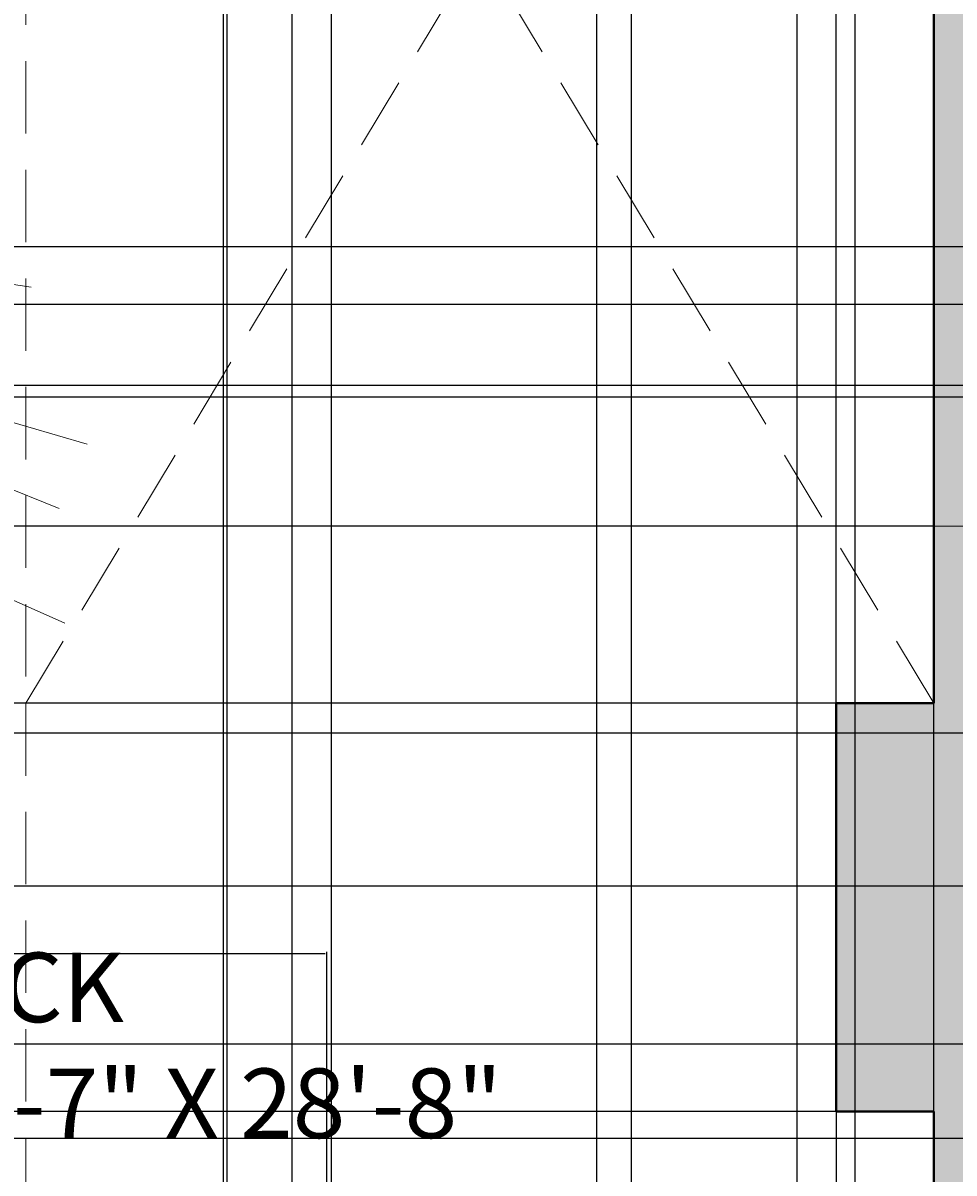
# Model space of a CAD drawing. Units: inches. Extents: x 818 to 1898, y 976 to 2364.
# Tile 63 of 96: x 1180 to 1260, y 1873 to 1972. Entities that reach past the tile are written whole.
import ezdxf

# ---------------------------------------------------------------- set-up
doc = ezdxf.new("R2010")
doc.units = ezdxf.units.IN
doc.header["$LTSCALE"] = 5
doc.header["$MEASUREMENT"] = 0
doc.linetypes.add('HIDDEN', pattern=[0.375, 0.25, -0.125])
for name, color, linetype, lineweight in [('A-ANNO-DIMS', 2, 'Continuous', 18), ('A-AREA-IDEN', 7, 'Continuous', 18), ('A-FLOR-OVHD', 8, 'HIDDEN', 13), ('A-GLAZ', 4, 'Continuous', 18), ('A-WALL', 7, 'Continuous', 40)]:
    doc.layers.add(name, color=color, linetype=linetype, lineweight=lineweight)
for name, color, linetype, lineweight, true_color in [('A-GLAZ-PATT', 141, 'Continuous', 9, 0xadddf7), ('A-WALL-PATT', 251, 'Continuous', 13, 0x636466), ('L-PLNT', 116, 'Continuous', 13, 0x136734)]:
    doc.layers.add(name, color=color, linetype=linetype, lineweight=lineweight, true_color=true_color)
doc.styles.get("Standard").update_dxf_attribs({"font": 'arial.ttf'})
doc.dimstyles.get("Standard").update_dxf_attribs({"dimtxt": 0.18, "dimasz": 0.18, "dimexe": 0.18, "dimexo": 0.0625, "dimgap": 0.09, "dimtad": 0, "dimtih": 1, "dimtoh": 1, "dimdec": 4, "dimzin": 0, "dimdsep": 46, "dimtxsty": 'Standard', "dimcen": 0.09, "dimadec": 0, "dimazin": 0, "dimtfac": 1, "dimtdec": 4, "dimtofl": 0, "dimtmove": 0, "dimatfit": 3, "dimfxl": 1, "dimtolj": 1, "dimtzin": 0, "dimarcsym": 0})

# ---------------------------------------------------------------- blocks, each defined once
blk = doc.blocks.new('PALM-DECK')
for p, q in [((90.505, 49.71), (123.241, 44.773)), ((98.69, 39.836), (128.056, 31.195)), ((99.652, 36.132), (125.649, 25.64)), ((102.541, 26.258), (126.13, 15.766))]:
    blk.add_line(p, q)
blk = doc.blocks.new('*D29')
at = {"layer": 'A-ANNO-DIMS', "color": 0, "lineweight": -2, "ltscale": 5, "transparency": 16777216}
for p, q in [((1064.31, 1870.244), (1064.31, 1892.189)), ((1064.49, 1892.009), (1134.729, 1892.009)), ((1206.147, 1892.009), (1135.908, 1892.009)), ((1206.327, 1870.244), (1206.327, 1892.189))]:
    blk.add_line(p, q, dxfattribs=at)
at = {"layer": 'A-ANNO-DIMS', "color": 0, "ltscale": 5, "transparency": 16777216}
for points in [[(1064.49, 1892.039), (1064.49, 1891.979), (1064.31, 1892.009)], [(1206.147, 1892.039), (1206.147, 1891.979), (1206.327, 1892.009)]]:
    blk.add_solid(points, dxfattribs=at)
at = {"layer": 'Defpoints', "color": 0, "ltscale": 5, "transparency": 16777216}
for p in [(1206.327, 1892.009), (1064.31, 1870.181), (1206.327, 1870.181)]:
    blk.add_point(p, dxfattribs=at)
at = {"layer": 'A-ANNO-DIMS', "color": 0, "ltscale": 5, "transparency": 16777216, "insert": (1135.319, 1892.009), "char_height": 0.18, "attachment_point": 5}
blk.add_mtext('\\A1;142 TYP.', dxfattribs=at)
blk = doc.blocks.new('*D59')
at = {"layer": 'A-ANNO-DIMS', "color": 0, "lineweight": -2, "ltscale": 5, "transparency": 16777216}
for p, q in [((1251.643, 2300.393), (818.026, 2300.393)), ((818.206, 2300.213), (818.206, 1669.95)), ((818.206, 1039.323), (818.206, 1669.586)), ((896.051, 1039.143), (818.026, 1039.143))]:
    blk.add_line(p, q, dxfattribs=at)
at = {"layer": 'A-ANNO-DIMS', "color": 0, "ltscale": 5, "transparency": 16777216}
for points in [[(818.176, 2300.213), (818.236, 2300.213), (818.206, 2300.393)], [(818.176, 1039.323), (818.236, 1039.323), (818.206, 1039.143)]]:
    blk.add_solid(points, dxfattribs=at)
at = {"layer": 'Defpoints', "color": 0, "ltscale": 5, "transparency": 16777216}
for p in [(818.206, 2300.393), (1251.706, 2300.393), (896.114, 1039.143)]:
    blk.add_point(p, dxfattribs=at)
at = {"layer": 'A-ANNO-DIMS', "color": 0, "ltscale": 5, "transparency": 16777216, "insert": (818.206, 1669.768), "char_height": 0.18, "attachment_point": 5}
blk.add_mtext('\\A1;1261.2', dxfattribs=at)
blk = doc.blocks.new('*D61')
at = {"layer": 'A-ANNO-DIMS', "color": 0, "lineweight": -2, "ltscale": 5, "transparency": 16777216}
for p, q in [((1071.725, 1203.027), (1071.725, 2363.873)), ((1430.725, 1203.027), (1430.725, 2363.873)), ((1071.905, 2363.693), (1250.936, 2363.693)), ((1430.545, 2363.693), (1251.514, 2363.693))]:
    blk.add_line(p, q, dxfattribs=at)
at = {"layer": 'A-ANNO-DIMS', "color": 0, "ltscale": 5, "transparency": 16777216}
for points in [[(1071.905, 2363.723), (1071.905, 2363.663), (1071.725, 2363.693)], [(1430.545, 2363.723), (1430.545, 2363.663), (1430.725, 2363.693)]]:
    blk.add_solid(points, dxfattribs=at)
at = {"layer": 'Defpoints', "color": 0, "ltscale": 5, "transparency": 16777216}
for p in [(1430.725, 2363.693), (1071.725, 1202.964), (1430.725, 1202.964)]:
    blk.add_point(p, dxfattribs=at)
at = {"layer": 'A-ANNO-DIMS', "color": 0, "ltscale": 5, "transparency": 16777216, "insert": (1251.225, 2363.693), "char_height": 0.18, "attachment_point": 5}
blk.add_mtext('\\A1;359', dxfattribs=at)
blk = doc.blocks.new('*D64')
at = {"layer": 'A-ANNO-DIMS', "color": 0, "lineweight": -2, "ltscale": 5, "transparency": 16777216}
for p, q in [((1197.725, 1501.141), (1197.725, 2363.873)), ((1430.725, 1501.141), (1430.725, 2363.873)), ((1197.905, 2363.693), (1313.935, 2363.693)), ((1430.545, 2363.693), (1314.516, 2363.693))]:
    blk.add_line(p, q, dxfattribs=at)
at = {"layer": 'A-ANNO-DIMS', "color": 0, "ltscale": 5, "transparency": 16777216}
for points in [[(1197.905, 2363.723), (1197.905, 2363.663), (1197.725, 2363.693)], [(1430.545, 2363.723), (1430.545, 2363.663), (1430.725, 2363.693)]]:
    blk.add_solid(points, dxfattribs=at)
at = {"layer": 'Defpoints', "color": 0, "ltscale": 5, "transparency": 16777216}
for p in [(1430.725, 2363.693), (1197.725, 1501.078), (1430.725, 1501.078)]:
    blk.add_point(p, dxfattribs=at)
at = {"layer": 'A-ANNO-DIMS', "color": 0, "ltscale": 5, "transparency": 16777216, "insert": (1314.225, 2363.693), "char_height": 0.18, "attachment_point": 5}
blk.add_mtext('\\A1;233', dxfattribs=at)
blk = doc.blocks.new('*D74')
at = {"layer": 'A-ANNO-DIMS', "color": 0, "lineweight": -2, "ltscale": 5, "transparency": 16777216}
for p, q in [((1590.663, 1940.078), (818.026, 1940.078)), ((818.206, 1939.898), (818.206, 1925.76)), ((818.206, 1911.258), (818.206, 1925.396)), ((1590.663, 1911.078), (818.026, 1911.078))]:
    blk.add_line(p, q, dxfattribs=at)
at = {"layer": 'A-ANNO-DIMS', "color": 0, "ltscale": 5, "transparency": 16777216}
for points in [[(818.176, 1939.898), (818.236, 1939.898), (818.206, 1940.078)], [(818.176, 1911.258), (818.236, 1911.258), (818.206, 1911.078)]]:
    blk.add_solid(points, dxfattribs=at)
at = {"layer": 'Defpoints', "color": 0, "ltscale": 5, "transparency": 16777216}
for p in [(818.206, 1940.078), (1590.725, 1940.078), (1590.725, 1911.078)]:
    blk.add_point(p, dxfattribs=at)
at = {"layer": 'A-ANNO-DIMS', "color": 0, "ltscale": 5, "transparency": 16777216, "insert": (818.206, 1925.578), "char_height": 0.18, "attachment_point": 5}
blk.add_mtext('\\A1;29', dxfattribs=at)
blk = doc.blocks.new('*D82')
at = {"layer": 'A-ANNO-DIMS', "color": 0, "lineweight": -2, "ltscale": 5, "transparency": 16777216}
for p, q in [((1083.725, 1501.141), (1083.725, 2363.873)), ((1197.725, 1501.141), (1197.725, 2363.873)), ((1083.905, 2363.693), (1140.445, 2363.693)), ((1197.545, 2363.693), (1141.005, 2363.693))]:
    blk.add_line(p, q, dxfattribs=at)
at = {"layer": 'A-ANNO-DIMS', "color": 0, "ltscale": 5, "transparency": 16777216}
for points in [[(1083.905, 2363.723), (1083.905, 2363.663), (1083.725, 2363.693)], [(1197.545, 2363.723), (1197.545, 2363.663), (1197.725, 2363.693)]]:
    blk.add_solid(points, dxfattribs=at)
at = {"layer": 'Defpoints', "color": 0, "ltscale": 5, "transparency": 16777216}
for p in [(1197.725, 2363.693), (1083.725, 1501.078), (1197.725, 1501.078)]:
    blk.add_point(p, dxfattribs=at)
at = {"layer": 'A-ANNO-DIMS', "color": 0, "ltscale": 5, "transparency": 16777216, "insert": (1140.725, 2363.693), "char_height": 0.18, "attachment_point": 5}
blk.add_mtext('\\A1;114', dxfattribs=at)
blk = doc.blocks.new('*D83')
at = {"layer": 'A-ANNO-DIMS', "color": 0, "lineweight": -2, "ltscale": 5, "transparency": 16777216}
for p, q in [((1197.725, 1700.141), (1197.725, 2363.873)), ((1258.725, 1700.141), (1258.725, 2363.873)), ((1197.905, 2363.693), (1228.023, 2363.693)), ((1258.545, 2363.693), (1228.427, 2363.693))]:
    blk.add_line(p, q, dxfattribs=at)
at = {"layer": 'A-ANNO-DIMS', "color": 0, "ltscale": 5, "transparency": 16777216}
for points in [[(1197.905, 2363.723), (1197.905, 2363.663), (1197.725, 2363.693)], [(1258.545, 2363.723), (1258.545, 2363.663), (1258.725, 2363.693)]]:
    blk.add_solid(points, dxfattribs=at)
at = {"layer": 'Defpoints', "color": 0, "ltscale": 5, "transparency": 16777216}
for p in [(1258.725, 2363.693), (1197.725, 1700.078), (1258.725, 1700.078)]:
    blk.add_point(p, dxfattribs=at)
at = {"layer": 'A-ANNO-DIMS', "color": 0, "ltscale": 5, "transparency": 16777216, "insert": (1228.225, 2363.693), "char_height": 0.18, "attachment_point": 5}
blk.add_mtext('\\A1;61', dxfattribs=at)
blk = doc.blocks.new('*D85')
at = {"layer": 'A-ANNO-DIMS', "color": 0, "lineweight": -2, "ltscale": 5, "transparency": 16777216}
for p, q in [((1258.788, 2053.078), (1897.916, 2053.078)), ((1897.736, 2052.898), (1897.736, 1876.76)), ((1897.736, 1700.258), (1897.736, 1876.396)), ((1258.788, 1700.078), (1897.916, 1700.078))]:
    blk.add_line(p, q, dxfattribs=at)
at = {"layer": 'A-ANNO-DIMS', "color": 0, "ltscale": 5, "transparency": 16777216}
for points in [[(1897.706, 2052.898), (1897.766, 2052.898), (1897.736, 2053.078)], [(1897.706, 1700.258), (1897.766, 1700.258), (1897.736, 1700.078)]]:
    blk.add_solid(points, dxfattribs=at)
at = {"layer": 'Defpoints', "color": 0, "ltscale": 5, "transparency": 16777216}
for p in [(1258.725, 2053.078), (1897.736, 2053.078), (1258.725, 1700.078)]:
    blk.add_point(p, dxfattribs=at)
at = {"layer": 'A-ANNO-DIMS', "color": 0, "ltscale": 5, "transparency": 16777216, "insert": (1897.736, 1876.578), "char_height": 0.18, "attachment_point": 5}
blk.add_mtext('\\A1;353', dxfattribs=at)
blk = doc.blocks.new('*D95')
at = {"layer": 'A-ANNO-DIMS', "color": 0, "lineweight": -2, "ltscale": 5, "transparency": 16777216}
for p, q in [((1173.542, 1071.118), (1173.542, 2363.873)), ((1229.647, 1071.118), (1229.647, 2363.873)), ((1173.722, 2363.693), (1201.288, 2363.693)), ((1229.467, 2363.693), (1201.901, 2363.693))]:
    blk.add_line(p, q, dxfattribs=at)
at = {"layer": 'A-ANNO-DIMS', "color": 0, "ltscale": 5, "transparency": 16777216}
for points in [[(1173.722, 2363.723), (1173.722, 2363.663), (1173.542, 2363.693)], [(1229.467, 2363.723), (1229.467, 2363.663), (1229.647, 2363.693)]]:
    blk.add_solid(points, dxfattribs=at)
at = {"layer": 'Defpoints', "color": 0, "ltscale": 5, "transparency": 16777216}
for p in [(1229.647, 2363.693), (1173.542, 1071.055), (1229.647, 1071.055)]:
    blk.add_point(p, dxfattribs=at)
at = {"layer": 'A-ANNO-DIMS', "color": 0, "ltscale": 5, "transparency": 16777216, "insert": (1201.595, 2363.693), "char_height": 0.18, "attachment_point": 5}
blk.add_mtext('\\A1;56.1', dxfattribs=at)
blk = doc.blocks.new('*D96')
at = {"layer": 'A-ANNO-DIMS', "color": 0, "lineweight": -2, "ltscale": 5, "transparency": 16777216}
for p, q in [((1229.647, 1071.118), (1229.647, 2363.873)), ((1284.17, 1071.118), (1284.17, 2363.873)), ((1229.827, 2363.693), (1256.516, 2363.693)), ((1283.99, 2363.693), (1257.301, 2363.693))]:
    blk.add_line(p, q, dxfattribs=at)
at = {"layer": 'A-ANNO-DIMS', "color": 0, "ltscale": 5, "transparency": 16777216}
for points in [[(1229.827, 2363.723), (1229.827, 2363.663), (1229.647, 2363.693)], [(1283.99, 2363.723), (1283.99, 2363.663), (1284.17, 2363.693)]]:
    blk.add_solid(points, dxfattribs=at)
at = {"layer": 'Defpoints', "color": 0, "ltscale": 5, "transparency": 16777216}
for p in [(1284.17, 2363.693), (1229.647, 1071.055), (1284.17, 1071.055)]:
    blk.add_point(p, dxfattribs=at)
at = {"layer": 'A-ANNO-DIMS', "color": 0, "ltscale": 5, "transparency": 16777216, "insert": (1256.909, 2363.693), "char_height": 0.18, "attachment_point": 5}
blk.add_mtext('\\A1;54.52', dxfattribs=at)
blk = doc.blocks.new('*D109')
at = {"layer": 'A-ANNO-DIMS', "color": 0, "lineweight": -2, "ltscale": 5, "transparency": 16777216}
for p, q in [((1125.917, 1410.117), (1125.917, 2363.873)), ((1203.329, 1409.911), (1203.329, 2363.873)), ((1126.097, 2363.693), (1164.248, 2363.693)), ((1203.149, 2363.693), (1164.999, 2363.693))]:
    blk.add_line(p, q, dxfattribs=at)
at = {"layer": 'A-ANNO-DIMS', "color": 0, "ltscale": 5, "transparency": 16777216}
for points in [[(1126.097, 2363.723), (1126.097, 2363.663), (1125.917, 2363.693)], [(1203.149, 2363.723), (1203.149, 2363.663), (1203.329, 2363.693)]]:
    blk.add_solid(points, dxfattribs=at)
at = {"layer": 'Defpoints', "color": 0, "ltscale": 5, "transparency": 16777216}
for p in [(1203.329, 2363.693), (1125.917, 1410.055), (1203.329, 1409.848)]:
    blk.add_point(p, dxfattribs=at)
at = {"layer": 'A-ANNO-DIMS', "color": 0, "ltscale": 5, "transparency": 16777216, "insert": (1164.623, 2363.693), "char_height": 0.18, "attachment_point": 5}
blk.add_mtext('\\A1;77.41', dxfattribs=at)
blk = doc.blocks.new('*D121')
at = {"layer": 'A-ANNO-DIMS', "color": 0, "lineweight": -2, "ltscale": 5, "transparency": 16777216}
for p, q in [((1766.29, 1884.203), (818.026, 1884.203)), ((818.206, 1884.023), (818.206, 1841.142)), ((818.206, 1797.897), (818.206, 1840.778)), ((1766.29, 1797.717), (818.026, 1797.717))]:
    blk.add_line(p, q, dxfattribs=at)
at = {"layer": 'A-ANNO-DIMS', "color": 0, "ltscale": 5, "transparency": 16777216}
for points in [[(818.176, 1884.023), (818.236, 1884.023), (818.206, 1884.203)], [(818.176, 1797.897), (818.236, 1797.897), (818.206, 1797.717)]]:
    blk.add_solid(points, dxfattribs=at)
at = {"layer": 'Defpoints', "color": 0, "ltscale": 5, "transparency": 16777216}
for p in [(818.206, 1884.203), (1766.352, 1884.203), (1766.352, 1797.717)]:
    blk.add_point(p, dxfattribs=at)
at = {"layer": 'A-ANNO-DIMS', "color": 0, "ltscale": 5, "transparency": 16777216, "insert": (818.206, 1840.96), "char_height": 0.18, "attachment_point": 5}
blk.add_mtext('\\A1;86.49', dxfattribs=at)
blk = doc.blocks.new('*D145')
at = {"layer": 'A-ANNO-DIMS', "color": 0, "lineweight": -2, "ltscale": 5, "transparency": 16777216}
for p, q in [((1197.393, 2122.314), (1197.393, 975.663)), ((1232.609, 2122.314), (1232.609, 975.663)), ((1197.573, 975.843), (1214.608, 975.843)), ((1232.429, 975.843), (1215.394, 975.843))]:
    blk.add_line(p, q, dxfattribs=at)
at = {"layer": 'A-ANNO-DIMS', "color": 0, "ltscale": 5, "transparency": 16777216}
for points in [[(1197.573, 975.873), (1197.573, 975.813), (1197.393, 975.843)], [(1232.429, 975.873), (1232.429, 975.813), (1232.609, 975.843)]]:
    blk.add_solid(points, dxfattribs=at)
at = {"layer": 'Defpoints', "color": 0, "ltscale": 5, "transparency": 16777216}
for p in [(1197.393, 2122.377), (1232.609, 2122.377), (1232.609, 975.843)]:
    blk.add_point(p, dxfattribs=at)
at = {"layer": 'A-ANNO-DIMS', "color": 0, "ltscale": 5, "transparency": 16777216, "insert": (1215.001, 975.843), "char_height": 0.18, "attachment_point": 5}
blk.add_mtext('\\A1;35.22', dxfattribs=at)
blk = doc.blocks.new('*D162')
at = {"layer": 'A-ANNO-DIMS', "color": 0, "lineweight": -2, "ltscale": 5, "transparency": 16777216}
for p, q in [((1429.163, 1876.078), (818.026, 1876.078)), ((818.206, 1875.898), (818.206, 1871.76)), ((818.206, 1867.258), (818.206, 1871.396)), ((1429.163, 1867.078), (818.026, 1867.078))]:
    blk.add_line(p, q, dxfattribs=at)
at = {"layer": 'A-ANNO-DIMS', "color": 0, "ltscale": 5, "transparency": 16777216}
for points in [[(818.176, 1875.898), (818.236, 1875.898), (818.206, 1876.078)], [(818.176, 1867.258), (818.236, 1867.258), (818.206, 1867.078)]]:
    blk.add_solid(points, dxfattribs=at)
at = {"layer": 'Defpoints', "color": 0, "ltscale": 5, "transparency": 16777216}
for p in [(1429.225, 1876.078), (818.206, 1867.078), (1429.225, 1867.078)]:
    blk.add_point(p, dxfattribs=at)
at = {"layer": 'A-ANNO-DIMS', "color": 0, "ltscale": 5, "transparency": 16777216, "insert": (818.206, 1871.578), "char_height": 0.18, "attachment_point": 5}
blk.add_mtext('\\A1;9', dxfattribs=at)
blk = doc.blocks.new('*D206')
at = {"layer": 'A-ANNO-DIMS', "color": 0, "lineweight": -2, "ltscale": 5, "transparency": 16777216}
for p, q in [((1590.663, 1911.078), (818.026, 1911.078)), ((818.206, 1910.898), (818.206, 1893.76)), ((818.206, 1876.258), (818.206, 1893.396)), ((1590.663, 1876.078), (818.026, 1876.078))]:
    blk.add_line(p, q, dxfattribs=at)
at = {"layer": 'A-ANNO-DIMS', "color": 0, "ltscale": 5, "transparency": 16777216}
for points in [[(818.176, 1910.898), (818.236, 1910.898), (818.206, 1911.078)], [(818.176, 1876.258), (818.236, 1876.258), (818.206, 1876.078)]]:
    blk.add_solid(points, dxfattribs=at)
at = {"layer": 'Defpoints', "color": 0, "ltscale": 5, "transparency": 16777216}
for p in [(818.206, 1911.078), (1590.725, 1911.078), (1590.725, 1876.078)]:
    blk.add_point(p, dxfattribs=at)
at = {"layer": 'A-ANNO-DIMS', "color": 0, "ltscale": 5, "transparency": 16777216, "insert": (818.206, 1893.578), "char_height": 0.18, "attachment_point": 5}
blk.add_mtext('\\A1;35', dxfattribs=at)
blk = doc.blocks.new('*D211')
at = {"layer": 'A-ANNO-DIMS', "color": 0, "lineweight": -2, "ltscale": 5, "transparency": 16777216}
for p, q in [((1599.66265, 1948.078237), (818.025912, 1948.078237)), ((818.205912, 1947.898237), (818.205912, 1944.758237)), ((818.205912, 1941.258237), (818.205912, 1944.398237)), ((1599.66265, 1941.078237), (818.025912, 1941.078237))]:
    blk.add_line(p, q, dxfattribs=at)
at = {"layer": 'A-ANNO-DIMS', "color": 0, "ltscale": 5, "transparency": 16777216}
for points in [[(818.175912, 1947.898237), (818.235912, 1947.898237), (818.205912, 1948.078237)], [(818.175912, 1941.258237), (818.235912, 1941.258237), (818.205912, 1941.078237)]]:
    blk.add_solid(points, dxfattribs=at)
at = {"layer": 'Defpoints', "color": 0, "ltscale": 5, "transparency": 16777216}
for p in [(818.205912, 1948.078237), (1599.72515, 1948.078237), (1599.72515, 1941.078237)]:
    blk.add_point(p, dxfattribs=at)
at = {"layer": 'A-ANNO-DIMS', "color": 0, "ltscale": 5, "transparency": 16777216, "insert": (818.205912, 1944.578237), "char_height": 0.18, "attachment_point": 5}
blk.add_mtext('\\A1;7', dxfattribs=at)
blk = doc.blocks.new('*D215')
at = {"layer": 'A-ANNO-DIMS', "color": 0, "lineweight": -2, "ltscale": 5, "transparency": 16777216}
for p, q in [((1590.663, 1876.078), (818.026, 1876.078)), ((818.206, 1875.898), (818.206, 1781.76)), ((818.206, 1687.258), (818.206, 1781.396)), ((1511.663, 1687.078), (818.026, 1687.078))]:
    blk.add_line(p, q, dxfattribs=at)
at = {"layer": 'A-ANNO-DIMS', "color": 0, "ltscale": 5, "transparency": 16777216}
for points in [[(818.176, 1875.898), (818.236, 1875.898), (818.206, 1876.078)], [(818.176, 1687.258), (818.236, 1687.258), (818.206, 1687.078)]]:
    blk.add_solid(points, dxfattribs=at)
at = {"layer": 'Defpoints', "color": 0, "ltscale": 5, "transparency": 16777216}
for p in [(818.206, 1876.078), (1590.725, 1876.078), (1511.725, 1687.078)]:
    blk.add_point(p, dxfattribs=at)
at = {"layer": 'A-ANNO-DIMS', "color": 0, "ltscale": 5, "transparency": 16777216, "insert": (818.206, 1781.578), "char_height": 0.18, "attachment_point": 5}
blk.add_mtext('\\A1;189', dxfattribs=at)
blk = doc.blocks.new('*D232')
at = {"layer": 'A-ANNO-DIMS', "color": 0, "lineweight": -2, "ltscale": 5, "transparency": 16777216}
for p, q in [((1303.869, 2008.392), (818.026, 2008.392)), ((818.206, 2008.212), (818.206, 1980.898)), ((818.206, 1953.221), (818.206, 1980.534)), ((1303.869, 1953.041), (818.026, 1953.041))]:
    blk.add_line(p, q, dxfattribs=at)
at = {"layer": 'A-ANNO-DIMS', "color": 0, "ltscale": 5, "transparency": 16777216}
for points in [[(818.176, 2008.212), (818.236, 2008.212), (818.206, 2008.392)], [(818.176, 1953.221), (818.236, 1953.221), (818.206, 1953.041)]]:
    blk.add_solid(points, dxfattribs=at)
at = {"layer": 'Defpoints', "color": 0, "ltscale": 5, "transparency": 16777216}
for p in [(818.206, 2008.392), (1303.931, 2008.392), (1303.931, 1953.041)]:
    blk.add_point(p, dxfattribs=at)
at = {"layer": 'A-ANNO-DIMS', "color": 0, "ltscale": 5, "transparency": 16777216, "insert": (818.206, 1980.716), "char_height": 0.18, "attachment_point": 5}
blk.add_mtext('\\A1;55.35', dxfattribs=at)
blk = doc.blocks.new('*D248')
at = {"layer": 'A-ANNO-DIMS', "color": 0, "lineweight": -2, "ltscale": 5, "transparency": 16777216}
for p, q in [((1258.663, 2019.287), (818.026, 2019.287)), ((818.206, 2019.107), (818.206, 1974.286)), ((818.206, 1929.102), (818.206, 1973.922)), ((1258.663, 1928.922), (818.026, 1928.922))]:
    blk.add_line(p, q, dxfattribs=at)
at = {"layer": 'A-ANNO-DIMS', "color": 0, "ltscale": 5, "transparency": 16777216}
for points in [[(818.176, 2019.107), (818.236, 2019.107), (818.206, 2019.287)], [(818.176, 1929.102), (818.236, 1929.102), (818.206, 1928.922)]]:
    blk.add_solid(points, dxfattribs=at)
at = {"layer": 'Defpoints', "color": 0, "ltscale": 5, "transparency": 16777216}
for p in [(818.206, 2019.287), (1258.725, 2019.287), (1258.725, 1928.922)]:
    blk.add_point(p, dxfattribs=at)
at = {"layer": 'A-ANNO-DIMS', "color": 0, "ltscale": 5, "transparency": 16777216, "insert": (818.206, 1974.104), "char_height": 0.18, "attachment_point": 5}
blk.add_mtext('\\A1;90.37', dxfattribs=at)
blk = doc.blocks.new('*D250')
at = {"layer": 'A-ANNO-DIMS', "color": 0, "lineweight": -2, "ltscale": 5, "transparency": 16777216}
for p, q in [((1250.24, 1913.64), (818.026, 1913.64)), ((818.206, 1913.46), (818.206, 1896.198)), ((818.206, 1878.572), (818.206, 1895.834)), ((1250.24, 1878.392), (818.026, 1878.392))]:
    blk.add_line(p, q, dxfattribs=at)
at = {"layer": 'A-ANNO-DIMS', "color": 0, "ltscale": 5, "transparency": 16777216}
for points in [[(818.176, 1913.46), (818.236, 1913.46), (818.206, 1913.64)], [(818.176, 1878.572), (818.236, 1878.572), (818.206, 1878.392)]]:
    blk.add_solid(points, dxfattribs=at)
at = {"layer": 'Defpoints', "color": 0, "ltscale": 5, "transparency": 16777216}
for p in [(818.206, 1913.64), (1250.303, 1913.64), (1250.303, 1878.392)]:
    blk.add_point(p, dxfattribs=at)
at = {"layer": 'A-ANNO-DIMS', "color": 0, "ltscale": 5, "transparency": 16777216, "insert": (818.206, 1896.016), "char_height": 0.18, "attachment_point": 5}
blk.add_mtext('\\A1;35.25', dxfattribs=at)
blk = doc.blocks.new('*D251')
at = {"layer": 'A-ANNO-DIMS', "color": 0, "lineweight": -2, "ltscale": 5, "transparency": 16777216}
for p, q in [((1250.303, 1878.329), (1250.303, 975.663)), ((1258.725, 1878.329), (1258.725, 975.663)), ((1250.483, 975.843), (1254.121, 975.843)), ((1258.545, 975.843), (1254.907, 975.843))]:
    blk.add_line(p, q, dxfattribs=at)
at = {"layer": 'A-ANNO-DIMS', "color": 0, "ltscale": 5, "transparency": 16777216}
for points in [[(1250.483, 975.873), (1250.483, 975.813), (1250.303, 975.843)], [(1258.545, 975.873), (1258.545, 975.813), (1258.725, 975.843)]]:
    blk.add_solid(points, dxfattribs=at)
at = {"layer": 'Defpoints', "color": 0, "ltscale": 5, "transparency": 16777216}
for p in [(1250.303, 1878.392), (1258.725, 1878.392), (1258.725, 975.843)]:
    blk.add_point(p, dxfattribs=at)
at = {"layer": 'A-ANNO-DIMS', "color": 0, "ltscale": 5, "transparency": 16777216, "insert": (1254.514, 975.843), "char_height": 0.18, "attachment_point": 5}
blk.add_mtext('\\A1;8.422', dxfattribs=at)
blk = doc.blocks.new('*D269')
at = {"layer": 'A-ANNO-DIMS', "color": 0, "lineweight": -2, "ltscale": 5, "transparency": 16777216}
for p, q in [((1246.938, 1534.141), (1246.938, 2363.873)), ((1341.259, 1534.141), (1341.259, 2363.873)), ((1247.118, 2363.693), (1293.706, 2363.693)), ((1341.079, 2363.693), (1294.491, 2363.693))]:
    blk.add_line(p, q, dxfattribs=at)
at = {"layer": 'A-ANNO-DIMS', "color": 0, "ltscale": 5, "transparency": 16777216}
for points in [[(1247.118, 2363.723), (1247.118, 2363.663), (1246.938, 2363.693)], [(1341.079, 2363.723), (1341.079, 2363.663), (1341.259, 2363.693)]]:
    blk.add_solid(points, dxfattribs=at)
at = {"layer": 'Defpoints', "color": 0, "ltscale": 5, "transparency": 16777216}
for p in [(1341.259, 2363.693), (1246.938, 1534.078), (1341.259, 1534.078)]:
    blk.add_point(p, dxfattribs=at)
at = {"layer": 'A-ANNO-DIMS', "color": 0, "ltscale": 5, "transparency": 16777216, "insert": (1294.099, 2363.693), "char_height": 0.18, "attachment_point": 5}
blk.add_mtext('\\A1;94.32', dxfattribs=at)
blk = doc.blocks.new('*D271')
at = {"layer": 'A-ANNO-DIMS', "color": 0, "lineweight": -2, "ltscale": 5, "transparency": 16777216}
for p, q in [((1206.725, 1510.141), (1206.725, 2363.873)), ((1246.938, 1510.141), (1246.938, 2363.873)), ((1206.905, 2363.693), (1226.451, 2363.693)), ((1246.758, 2363.693), (1227.211, 2363.693))]:
    blk.add_line(p, q, dxfattribs=at)
at = {"layer": 'A-ANNO-DIMS', "color": 0, "ltscale": 5, "transparency": 16777216}
for points in [[(1206.905, 2363.723), (1206.905, 2363.663), (1206.725, 2363.693)], [(1246.758, 2363.723), (1246.758, 2363.663), (1246.938, 2363.693)]]:
    blk.add_solid(points, dxfattribs=at)
at = {"layer": 'Defpoints', "color": 0, "ltscale": 5, "transparency": 16777216}
for p in [(1246.938, 2363.693), (1206.725, 1510.078), (1246.938, 1510.078)]:
    blk.add_point(p, dxfattribs=at)
at = {"layer": 'A-ANNO-DIMS', "color": 0, "ltscale": 5, "transparency": 16777216, "insert": (1226.831, 2363.693), "char_height": 0.18, "attachment_point": 5}
blk.add_mtext('\\A1;40.21', dxfattribs=at)
blk = doc.blocks.new('*D276')
at = {"layer": 'A-ANNO-DIMS', "color": 0, "lineweight": -2, "ltscale": 5, "transparency": 16777216}
for p, q in [((1206.725, 1687.141), (1206.725, 2363.873)), ((1251.933, 1681.439), (1251.933, 2363.873)), ((1206.905, 2363.693), (1228.949, 2363.693)), ((1251.753, 2363.693), (1229.709, 2363.693))]:
    blk.add_line(p, q, dxfattribs=at)
at = {"layer": 'A-ANNO-DIMS', "color": 0, "ltscale": 5, "transparency": 16777216}
for points in [[(1206.905, 2363.723), (1206.905, 2363.663), (1206.725, 2363.693)], [(1251.753, 2363.723), (1251.753, 2363.663), (1251.933, 2363.693)]]:
    blk.add_solid(points, dxfattribs=at)
at = {"layer": 'Defpoints', "color": 0, "ltscale": 5, "transparency": 16777216}
for p in [(1251.933, 2363.693), (1206.725, 1687.078), (1251.933, 1681.376)]:
    blk.add_point(p, dxfattribs=at)
at = {"layer": 'A-ANNO-DIMS', "color": 0, "ltscale": 5, "transparency": 16777216, "insert": (1229.329, 2363.693), "char_height": 0.18, "attachment_point": 5}
blk.add_mtext('\\A1;45.21', dxfattribs=at)
blk = doc.blocks.new('*D281')
at = {"layer": 'A-ANNO-DIMS', "color": 0, "lineweight": -2, "ltscale": 5, "transparency": 16777216}
for p, q in [((1250.303, 1913.703), (1250.303, 2363.873)), ((1590.725, 2011.141), (1590.725, 2363.873)), ((1250.483, 2363.693), (1420.121, 2363.693)), ((1590.545, 2363.693), (1420.907, 2363.693))]:
    blk.add_line(p, q, dxfattribs=at)
at = {"layer": 'A-ANNO-DIMS', "color": 0, "ltscale": 5, "transparency": 16777216}
for points in [[(1250.483, 2363.723), (1250.483, 2363.663), (1250.303, 2363.693)], [(1590.545, 2363.723), (1590.545, 2363.663), (1590.725, 2363.693)]]:
    blk.add_solid(points, dxfattribs=at)
at = {"layer": 'Defpoints', "color": 0, "ltscale": 5, "transparency": 16777216}
for p in [(1590.725, 2363.693), (1590.725, 2011.078), (1250.303, 1913.64)]:
    blk.add_point(p, dxfattribs=at)
at = {"layer": 'A-ANNO-DIMS', "color": 0, "ltscale": 5, "transparency": 16777216, "insert": (1420.514, 2363.693), "char_height": 0.18, "attachment_point": 5}
blk.add_mtext('\\A1;340.4', dxfattribs=at)
blk = doc.blocks.new('*D287')
at = {"layer": 'A-ANNO-DIMS', "color": 0, "lineweight": -2, "ltscale": 5, "transparency": 16777216}
for p, q in [((1303.869, 1953.041), (818.026, 1953.041)), ((818.206, 1952.861), (818.206, 1925.635)), ((818.206, 1898.046), (818.206, 1925.272)), ((1310.963, 1897.866), (818.026, 1897.866))]:
    blk.add_line(p, q, dxfattribs=at)
at = {"layer": 'A-ANNO-DIMS', "color": 0, "ltscale": 5, "transparency": 16777216}
for points in [[(818.176, 1952.861), (818.236, 1952.861), (818.206, 1953.041)], [(818.176, 1898.046), (818.236, 1898.046), (818.206, 1897.866)]]:
    blk.add_solid(points, dxfattribs=at)
at = {"layer": 'Defpoints', "color": 0, "ltscale": 5, "transparency": 16777216}
for p in [(818.206, 1953.041), (1303.931, 1953.041), (1311.025, 1897.866)]:
    blk.add_point(p, dxfattribs=at)
at = {"layer": 'A-ANNO-DIMS', "color": 0, "ltscale": 5, "transparency": 16777216, "insert": (818.206, 1925.454), "char_height": 0.18, "attachment_point": 5}
blk.add_mtext('\\A1;55.17', dxfattribs=at)

msp = doc.modelspace()

# ---------------------------------------------------------------- hatches: boundary and pattern name
at = {"layer": 'A-GLAZ-PATT', "ltscale": 5}
h = msp.add_hatch(color=256, dxfattribs=at)
h.dxf.hatch_style = 1
h.paths.add_polyline_path([(1283.8183, 1504.5782), (1206.7251, 1504.5782), (1206.7251, 1501.0782), (1283.8183, 1501.0782)])
h.paths.add_polyline_path([(1283.8183, 1510.0782), (1206.7251, 1510.0782), (1206.7251, 1506.5782), (1283.8183, 1506.5782)])
h.paths.add_polyline_path([(1490.9163, 1355.0782), (1439.7252, 1355.0782), (1439.7252, 1409.0522), (1436.2252, 1409.0522), (1436.2252, 1351.5782), (1490.9163, 1351.5782)])
h.paths.add_polyline_path([(1434.2252, 1409.0522), (1430.7251, 1409.0522), (1430.7251, 1346.0782), (1435.0799, 1346.0782), (1435.0731, 1346.1152), (1435.1501, 1346.0782), (1490.9163, 1346.0782), (1490.9163, 1349.5782), (1434.2252, 1349.5782)])
h.paths.add_polyline_path([(1714.7252, 1545.0782), (1711.2252, 1545.0782), (1711.2252, 1521.0782), (1714.7252, 1521.0782)])
h.paths.add_polyline_path([(1709.2252, 1545.0782), (1705.7252, 1545.0782), (1705.7252, 1521.0782), (1709.2252, 1521.0782)])
h.paths.add_polyline_path([(1714.7252, 1687.0782), (1711.2252, 1687.0782), (1711.2252, 1649.9029), (1714.7252, 1649.9029)])
h.paths.add_polyline_path([(1709.2252, 1687.0782), (1705.7252, 1687.0782), (1705.7252, 1649.9029), (1709.2252, 1649.9029)])
h.paths.add_polyline_path([(1709.2252, 1745.5584), (1705.7252, 1745.5584), (1705.7252, 1717.3178), (1709.2252, 1717.3178)])
h.paths.add_polyline_path([(1714.7252, 1745.5584), (1711.2252, 1745.5584), (1711.2252, 1717.3178), (1714.7252, 1717.3178)])
h.paths.add_polyline_path([(1714.7252, 2014.5114), (1711.2252, 2014.5114), (1711.2252, 1962.0338), (1714.7252, 1962.0338)])
h.paths.add_polyline_path([(1709.2252, 2014.5114), (1705.7252, 2014.5114), (1705.7252, 1962.0338), (1709.2252, 1962.0338)])
h.paths.add_polyline_path([(1538.5155, 2047.5782), (1485.1216, 2047.5782), (1485.1216, 2044.0782), (1538.5155, 2044.0782)])
h.paths.add_polyline_path([(1538.5155, 2053.0782), (1485.1216, 2053.0782), (1485.1216, 2049.5782), (1538.5155, 2049.5782)])
h.paths.add_polyline_path([(1388.0315, 2047.5782), (1330.305, 2047.5782), (1330.305, 2044.0782), (1388.0315, 2044.0782)])
h.paths.add_polyline_path([(1388.0315, 2053.0782), (1330.305, 2053.0782), (1330.305, 2049.5782), (1388.0315, 2049.5782)])
h.paths.add_polyline_path([(1262.2252, 2019.2871), (1258.7251, 2019.2871), (1258.7251, 1928.9218), (1262.2252, 1928.9218)])
h.paths.add_polyline_path([(1267.7252, 2019.2871), (1264.2252, 2019.2871), (1264.2252, 1928.9218), (1267.7252, 1928.9218)])
h.paths.add_polyline_path([(1262.2252, 1862.9652), (1258.7251, 1862.9652), (1258.7251, 1814.9652), (1262.2252, 1814.9652)])
h.paths.add_polyline_path([(1267.7252, 1862.9652), (1264.2252, 1862.9652), (1264.2252, 1814.9652), (1267.7252, 1814.9652)])
h.paths.add_polyline_path([(1262.2252, 1755.3321), (1258.7251, 1755.3321), (1258.7251, 1707.3321), (1262.2252, 1707.3321)])
h.paths.add_polyline_path([(1267.7252, 1755.3321), (1264.2252, 1755.3321), (1264.2252, 1707.3321), (1267.7252, 1707.3321)])
h.paths.add_polyline_path([(1251.9333, 1692.5782), (1206.7251, 1692.5782), (1206.7251, 1687.0782), (1251.9333, 1687.0782)])
h.paths.add_polyline_path([(1251.9333, 1700.0782), (1206.7251, 1700.0782), (1206.7251, 1694.5782), (1251.9333, 1694.5782)])
at = {"layer": 'A-WALL-PATT', "ltscale": 5}
h = msp.add_hatch(color=256, dxfattribs=at)
h.dxf.hatch_style = 1
h.paths.add_polyline_path([(1267.7252, 1928.9218), (1258.7251, 1928.9218), (1258.7251, 1913.6401), (1250.3029, 1913.6401), (1250.3029, 1878.3919), (1258.7251, 1878.3919), (1258.7251, 1862.9652), (1267.7252, 1862.9652)])
h.paths.add_polyline_path([(1267.7252, 1814.9652), (1258.7251, 1814.9652), (1258.7251, 1755.3321), (1267.7252, 1755.3321)])
h.paths.add_polyline_path([(1463.7252, 1696.0782), (1267.7252, 1696.0782), (1267.7252, 1707.3321), (1258.7251, 1707.3321), (1258.7251, 1700.0782), (1251.9333, 1700.0782), (1251.9333, 1687.0782), (1463.7252, 1687.0782)])
h.paths.add_polyline_path([(1714.7252, 1717.3178), (1705.7252, 1717.3178), (1705.7252, 1696.0782), (1599.7251, 1696.0782), (1599.7251, 1790.0782), (1705.7252, 1790.0782), (1705.7252, 1785.6125), (1714.7252, 1785.6125), (1714.7252, 1827.2125), (1705.7252, 1827.2125), (1705.7252, 1802.0782), (1599.7251, 1802.0782), (1599.7251, 1867.0782), (1705.7252, 1867.0782), (1705.7252, 1857.2125), (1714.7252, 1857.2125), (1714.7252, 1930.0316), (1741.8409, 1930.0316), (1741.8409, 1935.0316), (1714.7252, 1935.0316), (1714.7252, 1957.0338), (1741.8409, 1957.0338), (1741.8409, 1962.0338), (1714.7252, 1962.0338), (1705.7252, 1962.0338), (1705.7252, 1948.0782), (1599.7251, 1948.0782), (1599.7251, 1981.0782), (1590.7251, 1981.0782), (1590.7251, 1941.0782), (1620.7252, 1941.0782), (1705.7252, 1941.0782), (1705.7252, 1876.0782), (1599.7251, 1876.0782), (1599.7251, 1911.0782), (1590.7251, 1911.0782), (1590.7251, 1876.0782), (1429.2251, 1876.0782), (1429.2251, 1867.0782), (1511.7251, 1867.0782), (1528.593, 1867.0782), (1595.7252, 1867.0782), (1595.7252, 1773.0782), (1520.7252, 1773.0782), (1520.7252, 1837.5823), (1532.593, 1837.5823), (1532.593, 1867.0782), (1528.593, 1867.0782), (1528.593, 1841.5823), (1511.7251, 1841.5823), (1511.7251, 1744.9714), (1520.7252, 1744.9714), (1520.7252, 1761.0782), (1595.7252, 1761.0782), (1595.7252, 1696.0782), (1520.7252, 1696.0782), (1520.7252, 1716.0454), (1511.7251, 1716.0454), (1511.7251, 1696.0782), (1511.7251, 1687.0782), (1714.7252, 1687.0782)])
h.paths.add_polyline_path([(1714.7252, 2053.0782), (1714.7252, 2081.1881), (1709.7252, 2081.1881), (1709.7252, 2053.0782), (1681.6446, 2053.0782), (1681.6446, 2081.1881), (1676.6446, 2081.1881), (1676.6446, 2053.0782), (1538.5155, 2053.0782), (1538.5155, 2044.0782), (1590.7251, 2044.0782), (1590.7251, 2011.0782), (1599.7251, 2011.0782), (1599.7251, 2044.0782), (1705.7252, 2044.0782), (1705.7252, 2014.5114), (1714.7252, 2014.5114)])
h.paths.add_polyline_path([(1485.1216, 2053.0782), (1422.02, 2053.0782), (1422.02, 2081.1881), (1413.02, 2081.1881), (1413.02, 2053.0782), (1399.6356, 2053.0782), (1399.6356, 2081.1881), (1390.6356, 2081.1881), (1390.6356, 2053.0782), (1388.0315, 2053.0782), (1388.0315, 2044.0782), (1416.2743, 2044.0782), (1485.1216, 2044.0782)])
h.paths.add_polyline_path([(1330.305, 2053.0782), (1258.7251, 2053.0782), (1258.7251, 2019.2871), (1267.7252, 2019.2871), (1267.7252, 2044.0782), (1330.305, 2044.0782)])
h.paths.add_polyline_path([(1258.7251, 2053.0782), (1214.6577, 2053.0782), (1214.6577, 2044.0782), (1258.7251, 2044.0782)])
h.paths.add_polyline_path([(1214.6577, 2053.0782), (1180.349, 2053.0782), (1180.349, 2044.0782), (1214.6577, 2044.0782)])
h.paths.add_polyline_path([(1714.7252, 1639.5782), (1741.8409, 1639.5782), (1741.8409, 1643.5782), (1714.7252, 1643.5782), (1714.7252, 1649.9029), (1705.7252, 1649.9029), (1705.7252, 1600.0782), (1477.7252, 1600.0782), (1477.7252, 1591.0782), (1520.7252, 1591.0782), (1616.7252, 1591.0782), (1616.7252, 1416.6857), (1622.7252, 1416.6857), (1622.7252, 1463.0782), (1624.7252, 1463.0782), (1624.7252, 1467.0782), (1622.7252, 1467.0782), (1622.7252, 1591.0782), (1705.7252, 1591.0782), (1705.7252, 1545.0782), (1714.7252, 1545.0782), (1741.8409, 1545.0782), (1741.8409, 1549.0782), (1714.7252, 1549.0782), (1714.7252, 1593.9175), (1737.8409, 1593.9175), (1737.8409, 1597.9175), (1714.7252, 1597.9175)])
h.paths.add_polyline_path([(1674.9024, 2060.7419), (1714.7045, 2060.7419), (1714.7045, 2073.1061), (1674.9024, 2073.1061)], flags=25)
h.paths.add_polyline_path([(1394.5468, 2061.6618), (1422.2344, 2061.6618), (1422.2344, 2074.0261), (1394.5468, 2074.0261)], flags=24)

# ---------------------------------------------------------------- linework, layer by layer
at = {"layer": 'A-FLOR-OVHD', "ltscale": 5}
for p, q in [((1258.7251, 1913.6401), (1180.349, 2044.0782)), ((1180.349, 2044.0782), (1180.349, 1913.6401)), ((1180.349, 1913.6401), (1258.7251, 2044.0782)), ((1180.349, 1913.6401), (1258.7251, 1913.6401)), ((1180.349, 1913.6401), (1180.349, 1688.0782))]:
    msp.add_line(p, q, dxfattribs=at)
at = {"layer": 'A-GLAZ'}
msp.add_line((1267.7252, 1928.9218), (1258.7251, 1928.9218), dxfattribs=at)
at = {"layer": 'A-WALL'}
for p, q in [((1258.7251, 2053.0782), (1258.7251, 1913.6401)), ((1258.7251, 1878.3919), (1258.7251, 1700.0782))]:
    msp.add_line(p, q, dxfattribs=at)
at = {"layer": 'A-WALL', "ltscale": 5}
msp.add_lwpolyline([(1258.7251, 1913.6401), (1250.3029, 1913.6401), (1250.3029, 1878.3919), (1258.7251, 1878.3919)], dxfattribs=at)

# ---------------------------------------------------------------- block references
at = {"layer": 'L-PLNT'}
msp.add_blockref('PALM-DECK', (1057.571, 1904.8049), dxfattribs=at)

# ---------------------------------------------------------------- texts
at = {"layer": 'A-AREA-IDEN', "ltscale": 5, "insert": (1167.8608, 1892.1161), "char_height": 6, "attachment_point": 1}
msp.add_mtext_dynamic_manual_height_columns('DECK\\P14\'-7" X 28\'-8"', width=118.992422, gutter_width=1, heights=[0], dxfattribs=at)

# ---------------------------------------------------------------- dimensions: what is measured, and where the dimension line sits
at = {"layer": 'A-ANNO-DIMS', "ltscale": 5}
for base, p1, p2, override, picture, middle in [((1430.7251, 2363.6929), (1071.7251, 1202.9642), (1430.7251, 1202.9642), {"dimdec": 0, "dimlfac": 1, "dimrnd": 0, "dimzin": 0, "dimdsep": 46, "dimlunit": 2}, '*D61', (1251.2251, 2363.6929)), ((1197.7251, 2363.6929), (1083.7251, 1501.0782), (1197.7251, 1501.0782), {"dimdec": 0, "dimlfac": 1, "dimrnd": 0, "dimzin": 0, "dimdsep": 46, "dimlunit": 2}, '*D82', (1140.7251, 2363.6929)), ((1203.3292, 2363.6929), (1125.9172, 1410.0547), (1203.3292, 1409.8484), {"dimdec": 2, "dimlfac": 1, "dimrnd": 0, "dimzin": 0, "dimdsep": 46, "dimlunit": 2}, '*D109', (1164.6232, 2363.6929)), ((1229.6474, 2363.6929), (1173.5418, 1071.0552), (1229.6474, 1071.0552), {"dimdec": 1, "dimlfac": 1, "dimrnd": 0, "dimzin": 0, "dimdsep": 46, "dimlunit": 2}, '*D95', (1201.5946, 2363.6929)), ((1430.7251, 2363.6929), (1197.7251, 1501.0782), (1430.7251, 1501.0782), {"dimdec": 0, "dimlfac": 1, "dimrnd": 0, "dimzin": 0, "dimdsep": 46, "dimlunit": 2}, '*D64', (1314.2251, 2363.6929)), ((1258.7251, 2363.6929), (1197.7251, 1700.0782), (1258.7251, 1700.0782), {"dimdec": 0, "dimlfac": 1, "dimrnd": 0, "dimzin": 0, "dimdsep": 46, "dimlunit": 2}, '*D83', (1228.2251, 2363.6929)), ((1246.9377, 2363.6929), (1206.7251, 1510.0782), (1246.9377, 1510.0782), {"dimdec": 2, "dimlfac": 1, "dimrnd": 0, "dimzin": 0, "dimdsep": 46, "dimlunit": 2}, '*D271', (1226.8314, 2363.6929)), ((1251.9333, 2363.6929), (1206.7251, 1687.0782), (1251.9333, 1681.3763), {"dimdec": 2, "dimlfac": 1, "dimrnd": 0, "dimzin": 0, "dimdsep": 46, "dimlunit": 2}, '*D276', (1229.3292, 2363.6929)), ((1284.1697, 2363.6929), (1229.6474, 1071.0552), (1284.1697, 1071.0552), {"dimdec": 2, "dimlfac": 1, "dimrnd": 0, "dimzin": 0, "dimdsep": 46, "dimlunit": 2}, '*D96', (1256.9085, 2363.6929)), ((1341.2593, 2363.6929), (1246.9377, 1534.0782), (1341.2593, 1534.0782), {"dimdec": 2, "dimlfac": 1, "dimrnd": 0, "dimzin": 0, "dimdsep": 46, "dimlunit": 2}, '*D269', (1294.0985, 2363.6929)), ((1590.7251, 2363.6929), (1250.3029, 1913.6401), (1590.7251, 2011.0782), {"dimdec": 1, "dimlfac": 1, "dimrnd": 0, "dimzin": 0, "dimdsep": 46, "dimlunit": 2}, '*D281', (1420.514, 2363.6929)), ((1232.6091, 975.8433), (1197.3925, 2122.3767), (1232.6091, 2122.3767), {"dimdec": 2, "dimlfac": 1, "dimrnd": 0, "dimzin": 0, "dimdsep": 46, "dimlunit": 2}, '*D145', (1215.0008, 975.8433)), ((1258.7251, 975.8433), (1250.3029, 1878.3919), (1258.7251, 1878.3919), {"dimdec": 3, "dimlfac": 1, "dimrnd": 0, "dimzin": 0, "dimdsep": 46, "dimlunit": 2}, '*D251', (1254.514, 975.8433))]:
    dim = msp.add_linear_dim(base=base, p1=p1, p2=p2, dimstyle='Standard', override=override, dxfattribs=at)
    dim.commit()
    dim.dimension.update_dxf_attribs({"geometry": picture, "text_midpoint": middle})
for base, p1, p2, override, picture, middle in [((818.2059, 2300.3929), (896.1138, 1039.1433), (1251.7057, 2300.3929), {"dimdec": 1, "dimlfac": 1, "dimrnd": 0, "dimzin": 0, "dimdsep": 46, "dimlunit": 2}, '*D59', (818.2059, 1669.7681)), ((1897.736, 2053.0782), (1258.7251, 1700.0782), (1258.7251, 2053.0782), {"dimdec": 0, "dimlfac": 1, "dimrnd": 0, "dimzin": 0, "dimdsep": 46, "dimlunit": 2}, '*D85', (1897.736, 1876.5782)), ((818.2059, 2019.2871), (1258.7251, 1928.9218), (1258.7251, 2019.2871), {"dimdec": 2, "dimlfac": 1, "dimrnd": 0, "dimzin": 0, "dimdsep": 46, "dimlunit": 2}, '*D248', (818.2059, 1974.1044)), ((818.2059, 2008.3917), (1303.9314, 1953.0408), (1303.9314, 2008.3917), {"dimdec": 2, "dimlfac": 1, "dimrnd": 0, "dimzin": 0, "dimdsep": 46, "dimlunit": 2}, '*D232', (818.2059, 1980.7163)), ((818.2059, 1953.0408), (1311.025, 1897.8663), (1303.9314, 1953.0408), {"dimdec": 2, "dimlfac": 1, "dimrnd": 0, "dimzin": 0, "dimdsep": 46, "dimlunit": 2}, '*D287', (818.2059, 1925.4536)), ((818.2059, 1948.0782), (1599.7251, 1941.0782), (1599.7251, 1948.0782), {"dimdec": 0, "dimlfac": 1, "dimrnd": 0, "dimzin": 0, "dimdsep": 46, "dimlunit": 2}, '*D211', (818.2059, 1944.5782)), ((818.2059, 1940.0782), (1590.7251, 1911.0782), (1590.7251, 1940.0782), {"dimdec": 0, "dimlfac": 1, "dimrnd": 0, "dimzin": 0, "dimdsep": 46, "dimlunit": 2}, '*D74', (818.2059, 1925.5782)), ((818.2059, 1913.6401), (1250.3029, 1878.3919), (1250.3029, 1913.6401), {"dimdec": 2, "dimlfac": 1, "dimrnd": 0, "dimzin": 0, "dimdsep": 46, "dimlunit": 2}, '*D250', (818.2059, 1896.016)), ((818.2059, 1911.0782), (1590.7251, 1876.0782), (1590.7251, 1911.0782), {"dimdec": 0, "dimlfac": 1, "dimrnd": 0, "dimzin": 0, "dimdsep": 46, "dimlunit": 2}, '*D206', (818.2059, 1893.5782)), ((818.2059, 1884.2031), (1766.3524, 1797.7165), (1766.3524, 1884.2031), {"dimdec": 2, "dimlfac": 1, "dimrnd": 0, "dimzin": 0, "dimdsep": 46, "dimlunit": 2}, '*D121', (818.2059, 1840.9598)), ((818.2059, 1876.0782), (1511.7251, 1687.0782), (1590.7251, 1876.0782), {"dimdec": 0, "dimlfac": 1, "dimrnd": 0, "dimzin": 0, "dimdsep": 46, "dimlunit": 2}, '*D215', (818.2059, 1781.5782)), ((818.2059, 1867.0782), (1429.2251, 1876.0782), (1429.2251, 1867.0782), {"dimdec": 0, "dimlfac": 1, "dimrnd": 0, "dimzin": 0, "dimdsep": 46, "dimlunit": 2}, '*D162', (818.2059, 1871.5782))]:
    dim = msp.add_linear_dim(base=base, p1=p1, p2=p2, angle=90, dimstyle='Standard', override=override, dxfattribs=at)
    dim.commit()
    dim.dimension.update_dxf_attribs({"geometry": picture, "text_midpoint": middle})
dim = msp.add_linear_dim(base=(1206.3272, 1892.009), p1=(1064.3101, 1870.1814), p2=(1206.3272, 1870.1814), text='<> TYP.', dimstyle='Standard', override={"dimdec": 0, "dimlfac": 1, "dimrnd": 0, "dimzin": 0, "dimdsep": 46, "dimlunit": 2}, dxfattribs=at)
dim.commit()
dim.dimension.update_dxf_attribs({"geometry": '*D29', "text_midpoint": (1135.3187, 1892.009)})

doc.saveas('drawing.dxf')
